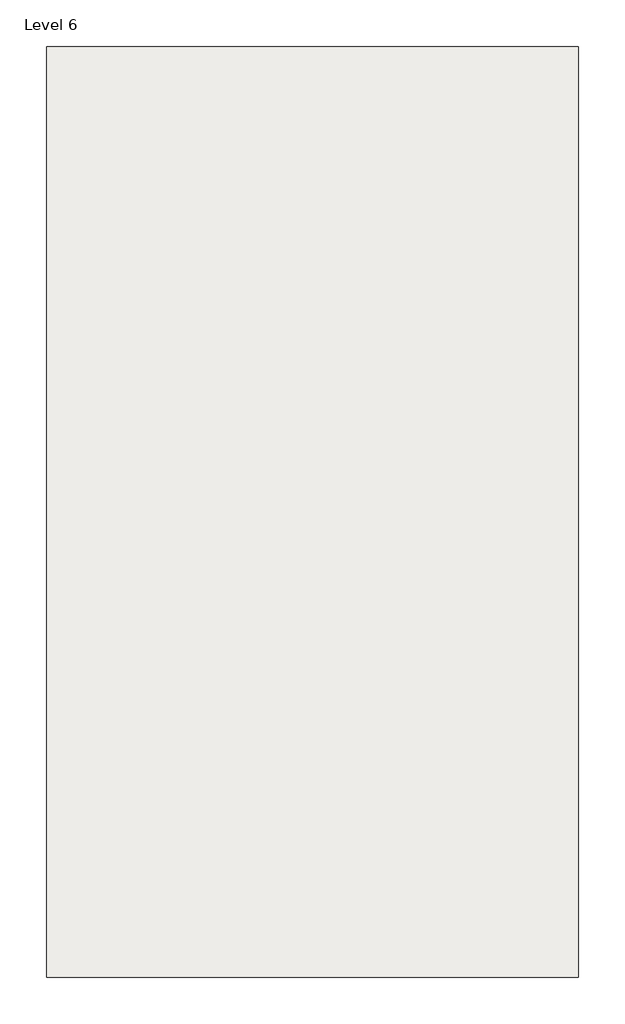
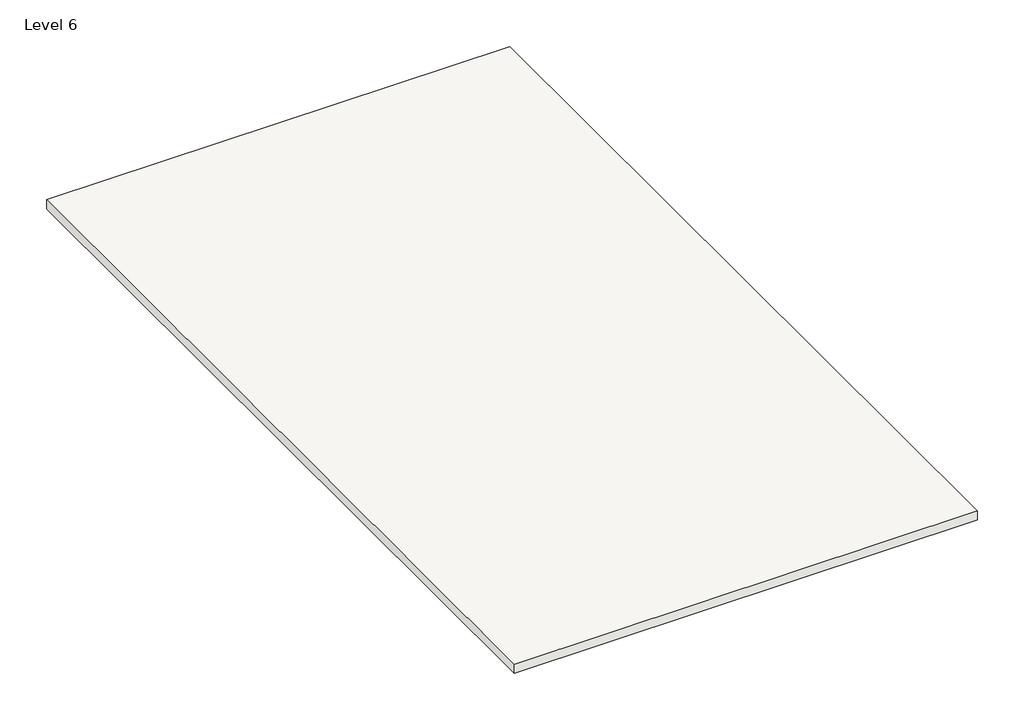
# One storey, incomplete: 1 roof.
"""IFC4 building model written with IfcOpenShell, lengths in millimetres."""

from ifc_helpers import new_model, si_unit, frame, origin, place, context, project, spatial, polyline, outline, extrude, element, save

model = new_model("IFC4")

# Units and contexts
model_context = context("Model", 3, world=origin())
ifc_project = project(units=[si_unit("LENGTHUNIT", "METRE", prefix="MILLI")], contexts=[model_context])

# Site, building, storey
site = spatial("IfcSite", under=ifc_project)
building = spatial("IfcBuilding", under=site)
storey = spatial("IfcBuildingStorey", under=building, Name="Level 6", Elevation=12801.6)

# Roof
placement = place(None, origin())
element("IfcRoof", 1, ObjectType="Generic - 12\"", at=placement, inside=storey, context=model_context, shape_type="SweptSolid", body=[
    extrude(outline(polyline([(-4881.0915084, 7034.2435985), (2370.6084916, 7034.2435985), (2370.6084916, -5653.0564015), (-4881.0915084, -5653.0564015), (-4881.0915084, 7034.2435985)])), frame((0.0, 0.0, 12649.2), z_axis=(0.0, 0.0, 1.0), x_axis=(1.0, 0.0, 0.0)), (0.0, 0.0, 1.0), 152.4),
])

save(model, "model.ifc")

# Revit data of these elements
# Type "Generic - 12\""
#   Assembly Code = "B1020"
#   Layers, outside or top first: 0' - 6" no material (function 1)
# Element 1 (IfcRoof, "Generic - 12\"")
#   built-in parameter 1001705 = 42 (stored number, unit not read)
#   built-in parameter 1001701 = -0.5 (stored number, unit not read)
#   built-in parameter 1001710 = 33615
#   Phase Created = New Construction
#   Materials on its faces: "Default Roof"
# Materials
#   "Default Roof": colour RGB 88 101 114, transparency 0, Cost = 0
